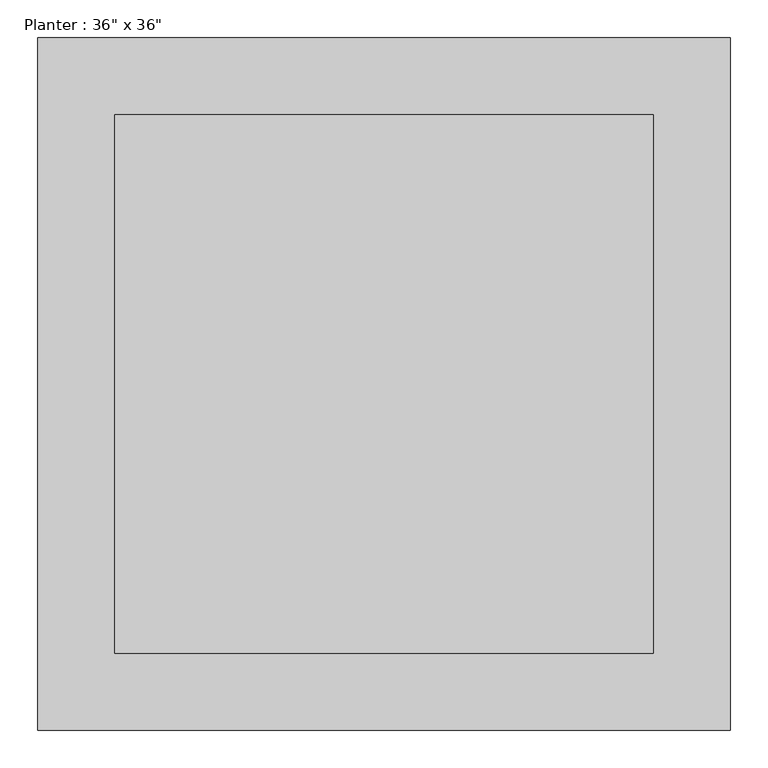
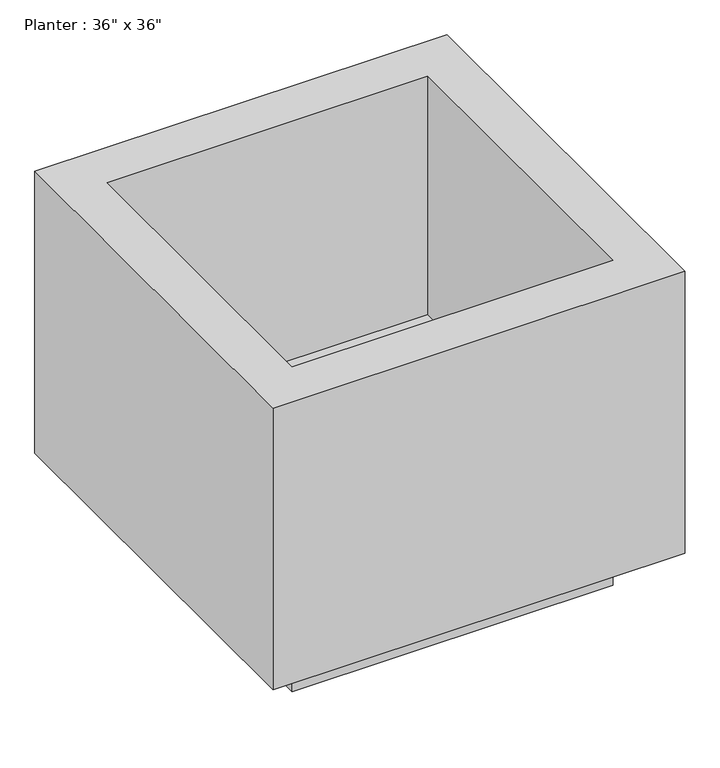
"""IFC4 building model written with IfcOpenShell, lengths in millimetres: geographic element geometry."""

from ifc_helpers import new_model, si_unit, origin, origin_with_axes, place, context, project, spatial, polyline, outline, extrude, faceted_brep, source, transform, mapped, element, save


def geographic_element_4c884dac(model_context):
    return source(origin(), model_context, "Body", "SolidModel", [
        extrude(outline(polyline([(355.6, 355.6), (355.6, -355.6), (-355.6, -355.6), (-355.6, 355.6), (355.6, 355.6)])), origin_with_axes(), (0.0, 0.0, 1.0), 101.6),
        faceted_brep([(457.2, 457.2, 762.0), (-457.2, 457.2, 762.0), (-457.2, -457.2, 762.0), (457.2, -457.2, 762.0), (-355.6, 355.6, 762.0), (355.6, 355.6, 762.0), (355.6, -355.6, 762.0), (-355.6, -355.6, 762.0), (457.2, 457.2, 101.6), (457.2, -457.2, 101.6), (-457.2, -457.2, 101.6), (-457.2, 457.2, 101.6), (355.6, 355.6, 203.2), (-355.6, 355.6, 203.2), (-355.6, -355.6, 203.2), (355.6, -355.6, 203.2)], [[[0, 1, 2, 3], [4, 5, 6, 7]], [[8, 9, 10, 11]], [[1, 0, 8, 11]], [[2, 1, 11, 10]], [[3, 2, 10, 9]], [[0, 3, 9, 8]], [[12, 13, 14, 15]], [[13, 12, 5, 4]], [[14, 13, 4, 7]], [[15, 14, 7, 6]], [[12, 15, 6, 5]]]),
    ])


if __name__ == "__main__":
    model = new_model("IFC4")
    model_context = context("Model", 3, world=origin())
    ifc_project = project(units=[si_unit("LENGTHUNIT", "METRE", prefix="MILLI")], contexts=[model_context])
    site = spatial("IfcSite", under=ifc_project)
    building = spatial("IfcBuilding", under=site)
    placement = place(None, origin())
    geographic_element_shape = geographic_element_4c884dac(model_context)
    element("IfcGeographicElement", 1, ObjectType="Planter : 36\" x 36\"", at=placement, inside=building, context=model_context, shape_type="MappedRepresentation", body=[
        mapped(geographic_element_shape, transform((0.0, 0.0, 0.0), x_axis=(1.0, 0.0, 0.0), y_axis=(0.0, 1.0, 0.0), z_axis=(0.0, 0.0, 1.0))),
    ])
    save(model, "model.ifc")

# Revit data of these elements
# Type "Planter : 36\" x 36\""
#   Depth = 3' - 0"
#   Height = 2' - 6"
#   Width = 3' - 0"
#   Material = Concrete, Precast
# Element 1 (IfcGeographicElement, "Planter : 36\" x 36\"")
#   Materials on its faces: "Concrete, Precast"
# Materials
#   "Concrete, Precast": class "Concrete", colour RGB 198 187 187, transparency 0, Description = "Precast concrete", Cost = 0
